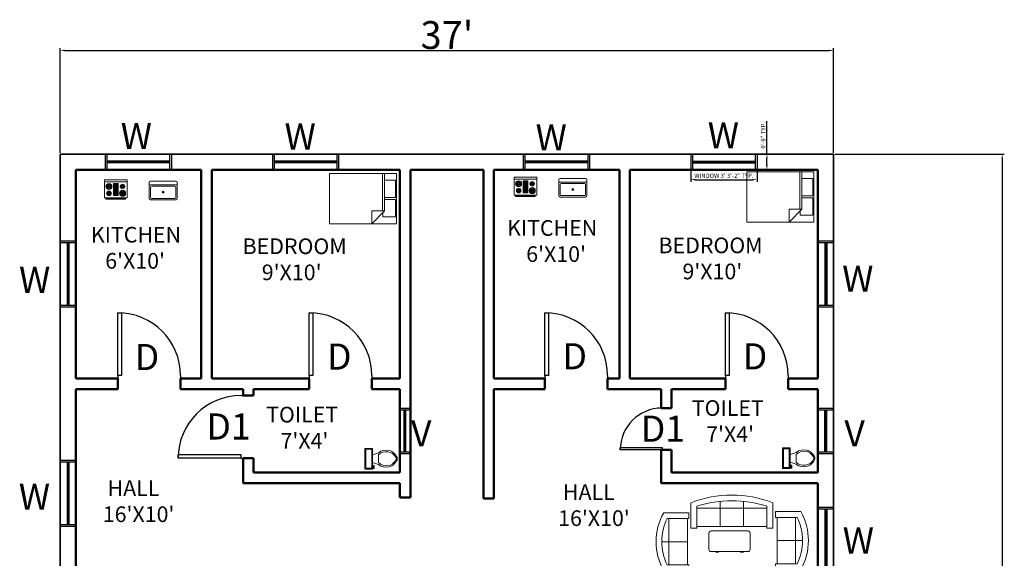
# Model space of a CAD drawing. Units: inches. Extents: x -25308 to -23933, y 10755 to 11996.
# Tile 4 of 6: x -25305 to -24739, y 11683 to 11992. Entities that reach past the tile are written whole.
import ezdxf

# ---------------------------------------------------------------- set-up
doc = ezdxf.new("R2010")
doc.units = ezdxf.units.IN
for name, color, linetype, lineweight in [('A-ANNO-DIMS', 2, 'Continuous', 18), ('A-ANNO-SYMB', 3, 'Continuous', 18), ('A-AREA-IDEN', 7, 'Continuous', 18), ('A-DOOR', 3, 'Continuous', 25), ('A-FLOR-FIXT', 8, 'Continuous', 18), ('A-FURN', 8, 'Continuous', 18), ('A-GLAZ', 4, 'Continuous', 25), ('A-WALL', 7, 'Continuous', 50), ('C-PROP', 30, 'Continuous', 35)]:
    doc.layers.add(name, color=color, linetype=linetype, lineweight=lineweight)
doc.styles.get("Standard").update_dxf_attribs({"font": 'arial.ttf'})
doc.dimstyles.new('ISO-25', dxfattribs={"dimtxt": 2.5, "dimasz": 2.5, "dimexe": 1.25, "dimexo": 0.625, "dimtad": 1, "dimdec": 0, "dimlunit": 3, "dimtxsty": 'Standard', "dimcen": 2.5, "dimadec": 0, "dimazin": 0, "dimtfac": 1, "dimtdec": 0, "dimtmove": 0, "dimatfit": 3, "dimfxl": 1, "dimarcsym": 0})

# ---------------------------------------------------------------- blocks, each defined once
blk = doc.blocks.new('*U8')
for p, q in [((0, 0), (0, -100)), ((750, 0), (750, -100))]:
    blk.add_line(p, q)
blk.add_lwpolyline([(0, 0), (0, 750), (43.75, 750), (43.75, 0)], close=True)
blk.add_arc((0, 0), 750, 0, 90)
blk = doc.blocks.new('Desk - 30 x 60 in.')
for p, q in [((-26.999995, 0), (26.999995, 0)), ((-29.999995, -27), (-29.999995, -3)), ((29.999995, -3), (29.999995, -27)), ((26.999995, -30), (-26.999995, -30)), ((-20.000005, -30), (-20.000005, -31)), ((-20.000005, -31), (-16.000005, -31)), ((-16.000005, -31), (-16.000005, -30)), ((15.999995, -31), (15.999995, -30)), ((19.999995, -31), (15.999995, -31)), ((19.999995, -30), (19.999995, -31))]:
    blk.add_line(p, q)
for centre, start, end in [((-26.499995, -3.5), 98.1301, 171.8699), ((26.499995, -3.5), 8.130102, 81.8699), ((-26.499995, -26.5), 188.1301, 261.8699), ((26.499995, -26.5), 278.1301, 351.8699)]:
    blk.add_arc(centre, 3.535534, start, end)
blk = doc.blocks.new('Sofa - Roundback 7 ft.')
for p, q in [((-12.00002, -32.4421), (-12.00003, -6.5971)), ((11.99997, -32.4421), (11.99998, -6.5971)), ((-36.000027, -34), (-36.000027, -11.4696)), ((-35.999844, -13.3819), (35.9998, -13.3819)), ((35.99998, -34), (35.99998, -11.4696)), ((-36.000027, -32.4421), (35.99998, -32.4421))]:
    blk.add_line(p, q)
for points in [[(-36.000027, -34), (-42.000027, -34), (-42.000027, -8)], [(41.99998, -8), (41.99998, -34), (35.99998, -34)]]:
    blk.add_lwpolyline(points)
for centre, radius, start, end in [((0, -114.25), 114.25, 68.43141, 111.5686), ((-0.00001, -127.1968), 121.1968, 72.72033, 107.2797)]:
    blk.add_arc(centre, radius, start, end)
blk = doc.blocks.new('Sofa - Roundback Loveseat 5 ft.')
for p, q in [((0, -32.44198), (0, -5.99998)), ((-24, -33.99998), (-24, -11.46958)), ((-23.9998, -13.38178), (23.99986, -13.38178)), ((24.00004, -33.99998), (24.00004, -11.46958)), ((-24, -32.44198), (24.00004, -32.44198))]:
    blk.add_line(p, q)
for points in [[(-24, -33.99998), (-30, -33.99998), (-30, -7.99998)], [(30.00004, -7.99998), (30.00004, -33.99998), (24.00004, -33.99998)]]:
    blk.add_lwpolyline(points)
for centre, radius, start, end in [((0, -60.24998), 60.24998, 60.13715, 119.8628), ((0, -61.38438), 55.38444, 64.32083, 115.6792)]:
    blk.add_arc(centre, radius, start, end)
blk = doc.blocks.new('Bed - Queen')
for p, q in [((0, -80.00003), (0, 0)), ((0, 0), (59.99999, 0)), ((59.99999, 0), (59.99999, -80.00003)), ((7.99999, -1.2), (28.79998, -1.2)), ((7.99999, -14.4), (7.99999, -1.2)), ((28.79998, -1.2), (28.79998, -14.4)), ((31.19999, -1.2), (51.99999, -1.2)), ((31.19999, -14.4), (31.19999, -1.2)), ((51.99999, -1.2), (51.99999, -16.4)), ((0, -14.4), (44.8, -14.4)), ((44.8, -16.8), (0, -16.8)), ((59.99999, -29.6), (44.8, -14.4)), ((44.8, -14.4), (44.8, -29.6)), ((51.99999, -16.4), (46.79936, -16.4)), ((44.8, -29.6), (59.99999, -29.6)), ((59.99999, -80.00003), (0, -80.00003))]:
    blk.add_line(p, q)
blk = doc.blocks.new('Range-Oven - 30 in top')
for p, q in [((0, -3), (30, -3)), ((12, -6), (18, -6)), ((13, -20), (13, -6)), ((14, -6), (14, -20)), ((15, -20), (15, -6)), ((16, -6), (16, -20)), ((17, -20), (17, -6)), ((6, -24), (6, -25)), ((8, -25), (8, -24)), ((18, -20), (12, -20)), ((22, -25), (22, -24)), ((24, -24), (24, -25))]:
    blk.add_line(p, q)
for points in [[(0, -24), (0, 0), (30, 0), (30, -24)], [(12, -21), (12, -5), (18, -5), (18, -21)], [(2, -26), (2, -25), (28, -25), (28, -26)]]:
    blk.add_lwpolyline(points, close=True)
for centre, radius in [((6, -9), 4), ((6, -9), 3), ((6, -9), 2), ((6, -9), 1), ((24, -9), 3), ((24, -9), 2), ((24, -9), 1), ((6, -18), 3), ((6, -18), 2), ((6, -18), 1), ((24, -18), 4), ((24, -18), 3), ((24, -18), 2), ((24, -18), 1)]:
    blk.add_circle(centre, radius)
blk = doc.blocks.new('Sink-single - 30 in top')
blk.add_line((-15, -3.999996), (15, -3.999996))
for points in [[(-13.5, 0), (13.5, 0)], [(-15, -18.499996), (-15, -1.5)], [(-13.5, -17.499996), (-13.5, -6.499996)], [(-12.5, -5.499996), (12.5, -5.499996)], [(13.5, -6.499996), (13.5, -17.499996)], [(15, -1.5), (15, -18.499996)], [(13.5, -19.999996), (-13.5, -19.999996)], [(12.5, -18.499996), (-12.5, -18.499996)]]:
    blk.add_lwpolyline(points)
for radius in [1, 0.5]:
    blk.add_circle((0, -11.999996), radius)
for centre, radius, start, end in [((-13.5, -1.5), 1.5, 90, 180), ((-12.5, -6.499996), 1, 90, 180), ((12.5, -6.499996), 1, 0, 90), ((13.5, -1.5), 1.5, 0, 90), ((-13.5, -18.499996), 1.5, 180, 270), ((-12.5, -17.499996), 1, 180, 270), ((12.5, -17.499996), 1, 270, 0), ((13.5, -18.499996), 1.5, 270, 0)]:
    blk.add_arc(centre, radius, start, end)
blk = doc.blocks.new('Toilet - top')
for p, q in [((-10, -8.5), (-8, -8.5)), ((-10, -9.5), (-10, -8.5)), ((-7, -9.5), (-10, -9.5)), ((-8, -8.5), (-8, -8)), ((-7, -8), (-7, -9.5)), ((-4, -8), (-6, -14)), ((4, -8), (6, -14)), ((9.5, -6), (9.5, -2)), ((4, -14), (-4, -14))]:
    blk.add_line(p, q)
blk.add_lwpolyline([(10.5, -8), (10.5, 0), (-10.5, 0), (-10.5, -8)], close=True)
for points in [[(-9.5, -2), (-9.5, -6)], [(8.5, -1), (-8.5, -1)], [(-8.5, -7), (8.5, -7)]]:
    blk.add_lwpolyline(points)
for centre, radius, start, end in [((-8.62, -1.88), 0.884, 81.8699, 188.1301), ((-8.62, -6.12), 0.884, 171.8699, 278.1301), ((8.62, -1.88), 0.884, 351.8699, 98.1301), ((8.62, -6.12), 0.884, 261.8699, 8.1301), ((3.52, -21.58), 12.17, 141.46911, 247.97143), ((4.2, -21.82), 11.33, 136.36773, 238.94682), ((-3.52, -21.58), 12.17, 292.02843, 38.53071), ((-4.2, -21.82), 11.33, 301.05301, 43.63209), ((0, -27.88), 4, 245.73182, 294.26817), ((0, -29), 4, 254.86053, 285.13947)]:
    blk.add_arc(centre, radius, start, end)
blk = doc.blocks.new('*D160')
at = {"layer": 'A-ANNO-DIMS', "color": 0, "lineweight": -2, "transparency": 16777216}
for p, q in [((-25281.44, 11915.75), (-25281.44, 11975.94)), ((-25278.94, 11974.69), (-24839.94, 11974.69)), ((-24837.44, 11915.75), (-24837.44, 11975.94))]:
    blk.add_line(p, q, dxfattribs=at)
at = {"layer": 'A-ANNO-DIMS', "color": 0, "transparency": 16777216}
for points in [[(-25278.94, 11975.11), (-25278.94, 11974.28), (-25281.44, 11974.69)], [(-24839.94, 11975.11), (-24839.94, 11974.28), (-24837.44, 11974.69)]]:
    blk.add_solid(points, dxfattribs=at)
at = {"layer": 'Defpoints', "color": 0, "transparency": 16777216}
for p in [(-24837.44, 11974.69), (-25281.44, 11915.12), (-24837.44, 11915.12)]:
    blk.add_point(p, dxfattribs=at)
at = {"layer": 'A-ANNO-DIMS', "color": 0, "transparency": 16777216, "insert": (-25059.44, 11983.49), "char_height": 2.5, "attachment_point": 5}
blk.add_mtext("{\\H6.4x;37'}", dxfattribs=at)
blk = doc.blocks.new('*D161')
at = {"layer": 'A-ANNO-DIMS', "color": 0, "lineweight": -2, "transparency": 16777216}
for p, q in [((-24836.82, 11915.12), (-24739.49, 11915.12)), ((-24740.74, 11912.62), (-24740.74, 10813.62)), ((-24836.82, 10811.12), (-24739.49, 10811.12))]:
    blk.add_line(p, q, dxfattribs=at)
at = {"layer": 'A-ANNO-DIMS', "color": 0, "transparency": 16777216}
for points in [[(-24741.15, 11912.62), (-24740.32, 11912.62), (-24740.74, 11915.12)], [(-24741.15, 10813.62), (-24740.32, 10813.62), (-24740.74, 10811.12)]]:
    blk.add_solid(points, dxfattribs=at)
at = {"layer": 'Defpoints', "color": 0, "transparency": 16777216}
for p in [(-24837.44, 11915.12), (-24837.44, 10811.12), (-24740.74, 10811.12)]:
    blk.add_point(p, dxfattribs=at)
at = {"layer": 'A-ANNO-DIMS', "color": 0, "transparency": 16777216, "insert": (-24749.53, 11363.12), "char_height": 2.5, "attachment_point": 5, "rotation": 90}
blk.add_mtext("{\\H6.4x;92'}", dxfattribs=at)
blk = doc.blocks.new('WIN-36-9IN')
for p, q in [((0, 9), (0, 0)), ((1, 9), (1, 0)), ((37, 9), (37, 0)), ((38, 9), (38, 0)), ((1, 5), (37, 5)), ((1, 4.5), (37, 4.5)), ((1, 4), (37, 4))]:
    blk.add_line(p, q)
blk = doc.blocks.new('VENT-24')
for p, q in [((0, 26), (9, 26)), ((0, 25), (9, 25)), ((4, 1), (4, 25)), ((4.5, 1), (4.5, 25)), ((5, 1), (5, 25)), ((0, 1), (9, 1)), ((0, 0), (9, 0))]:
    blk.add_line(p, q)
blk = doc.blocks.new('WIN-24-6IN')
for p, q in [((0, 26), (6, 26)), ((0, 25), (6, 25)), ((2.5, 1), (2.5, 25)), ((3, 1), (3, 25)), ((3.5, 1), (3.5, 25)), ((0, 1), (6, 1)), ((0, 0), (6, 0))]:
    blk.add_line(p, q)
blk = doc.blocks.new('*D182')
at = {"layer": 'A-ANNO-DIMS', "color": 0, "lineweight": -2, "transparency": 16777216}
for p, q in [((-24919.44, 11905.5), (-24919.44, 11899.17)), ((-24881.44, 11905.5), (-24881.44, 11899.17)), ((-24916.94, 11900.42), (-24883.94, 11900.42))]:
    blk.add_line(p, q, dxfattribs=at)
at = {"layer": 'A-ANNO-DIMS', "color": 0, "transparency": 16777216}
for points in [[(-24916.94, 11900.84), (-24916.94, 11900), (-24919.44, 11900.42)], [(-24883.94, 11900.84), (-24883.94, 11900), (-24881.44, 11900.42)]]:
    blk.add_solid(points, dxfattribs=at)
at = {"layer": 'Defpoints', "color": 0, "transparency": 16777216}
for p in [(-24919.44, 11906.12), (-24881.44, 11906.12), (-24881.44, 11900.42)]:
    blk.add_point(p, dxfattribs=at)
at = {"layer": 'A-ANNO-DIMS', "color": 0, "transparency": 16777216, "insert": (-24900.44, 11902.34), "char_height": 2.5, "attachment_point": 5}
blk.add_mtext('WINDOW 3\' 3\'-2" TYP.', dxfattribs=at)
blk = doc.blocks.new('*D183')
at = {"layer": 'A-ANNO-DIMS', "color": 0, "lineweight": -2, "transparency": 16777216}
for p, q in [((-24875.74, 11915.12), (-24875.74, 11934.11)), ((-24880.82, 11915.12), (-24874.49, 11915.12)), ((-24875.74, 11908.62), (-24875.74, 11912.62)), ((-24880.82, 11906.12), (-24874.49, 11906.12))]:
    blk.add_line(p, q, dxfattribs=at)
at = {"layer": 'A-ANNO-DIMS', "color": 0, "transparency": 16777216}
for points in [[(-24876.16, 11912.62), (-24875.33, 11912.62), (-24875.74, 11915.12)], [(-24876.16, 11908.62), (-24875.33, 11908.62), (-24875.74, 11906.12)]]:
    blk.add_solid(points, dxfattribs=at)
at = {"layer": 'Defpoints', "color": 0, "transparency": 16777216}
for p in [(-24881.44, 11915.12), (-24875.74, 11915.12), (-24881.44, 11906.12)]:
    blk.add_point(p, dxfattribs=at)
at = {"layer": 'A-ANNO-DIMS', "color": 0, "transparency": 16777216, "insert": (-24877.65, 11925.87), "char_height": 2.5, "attachment_point": 5, "rotation": 90}
blk.add_mtext('0\'-9" TYP.', dxfattribs=at)

msp = doc.modelspace()

# ---------------------------------------------------------------- linework, layer by layer
at = {"layer": 'A-WALL'}
for p, q in [((-25272.44, 11906.12), (-25200.44, 11906.12)), ((-25272.44, 11786.12), (-25272.44, 11906.12)), ((-25200.44, 11786.12), (-25200.44, 11906.12)), ((-25194.44, 11786.12), (-25194.44, 11906.12)), ((-25194.44, 11906.12), (-25086.44, 11906.12)), ((-25086.44, 11786.12), (-25086.44, 11906.12)), ((-25080.44, 11906.12), (-25038.44, 11906.12)), ((-25080.44, 11717.94), (-25080.44, 11906.12)), ((-25038.44, 11906.12), (-25038.44, 11717.22)), ((-25032.44, 11906.12), (-25032.44, 11786.12)), ((-25032.44, 11906.12), (-24960.44, 11906.12)), ((-24960.44, 11906.12), (-24960.44, 11786.12)), ((-24960.44, 11906.12), (-24960.44, 11786.12)), ((-24960.44, 11906.12), (-24960.44, 11786.12)), ((-24960.44, 11906.12), (-24960.44, 11786.12)), ((-24954.44, 11906.12), (-24954.44, 11786.12)), ((-24954.44, 11906.12), (-24954.44, 11786.12)), ((-24954.44, 11906.12), (-24954.44, 11786.12)), ((-24954.44, 11906.12), (-24954.44, 11786.12)), ((-24954.44, 11906.12), (-24846.44, 11906.12)), ((-24846.44, 11906.12), (-24846.44, 11786.12)), ((-25272.44, 11786.12), (-25248.38, 11786.12)), ((-25248.38, 11786.12), (-25248.38, 11780.12)), ((-25212.38, 11786.12), (-25212.38, 11780.12)), ((-25212.38, 11786.12), (-25200.44, 11786.12)), ((-25194.44, 11786.12), (-25138.54, 11786.12)), ((-25138.54, 11786.12), (-25138.54, 11780.12)), ((-25102.54, 11786.12), (-25102.54, 11780.12)), ((-25102.54, 11786.12), (-25086.44, 11786.12)), ((-25032.44, 11786.12), (-25003.22, 11786.12)), ((-25003.22, 11786.12), (-25003.22, 11780.12)), ((-24967.22, 11786.12), (-24967.22, 11780.12)), ((-24967.22, 11786.12), (-24960.44, 11786.12)), ((-24954.44, 11786.12), (-24899.58, 11786.12)), ((-24899.58, 11786.12), (-24899.58, 11780.12)), ((-24863.58, 11786.12), (-24863.58, 11780.12)), ((-24863.58, 11786.12), (-24846.44, 11786.12)), ((-25272.44, 11780.12), (-25248.38, 11780.12)), ((-25272.44, 11660.12), (-25272.44, 11780.12)), ((-25212.38, 11780.12), (-25176.44, 11780.12)), ((-25176.44, 11776.42), (-25176.44, 11780.12)), ((-25176.44, 11776.42), (-25176.44, 11780.12)), ((-25176.44, 11776.42), (-25176.44, 11780.12)), ((-25170.44, 11780.12), (-25138.54, 11780.12)), ((-25170.44, 11776.42), (-25170.44, 11780.12)), ((-25170.44, 11776.42), (-25170.44, 11780.12)), ((-25170.44, 11776.42), (-25170.44, 11780.12)), ((-25102.54, 11780.12), (-25086.44, 11780.12)), ((-25086.44, 11732.12), (-25086.44, 11780.12)), ((-25032.44, 11780.12), (-25003.22, 11780.12)), ((-25032.44, 11780.12), (-25032.44, 11717.22)), ((-24967.22, 11780.12), (-24936.44, 11780.12)), ((-24936.44, 11780.12), (-24936.44, 11769.19)), ((-24936.44, 11780.12), (-24936.44, 11769.19)), ((-24936.44, 11780.12), (-24936.44, 11769.19)), ((-24936.44, 11780.12), (-24936.44, 11769.19)), ((-24930.44, 11780.12), (-24930.44, 11769.19)), ((-24930.44, 11780.12), (-24930.44, 11769.19)), ((-24930.44, 11780.12), (-24930.44, 11769.19)), ((-24930.44, 11780.12), (-24930.44, 11769.19)), ((-24930.44, 11780.12), (-24899.58, 11780.12)), ((-24863.58, 11780.12), (-24846.44, 11780.12)), ((-24846.44, 11780.12), (-24846.44, 11732.12)), ((-25176.44, 11776.42), (-25170.44, 11776.42)), ((-24936.44, 11769.19), (-24930.44, 11769.19)), ((-24936.44, 11745.19), (-24930.44, 11745.19)), ((-24936.44, 11745.19), (-24936.44, 11726.12)), ((-24936.44, 11745.19), (-24936.44, 11726.12)), ((-24936.44, 11745.19), (-24936.44, 11726.12)), ((-24936.44, 11745.19), (-24936.44, 11726.12)), ((-24930.44, 11745.19), (-24930.44, 11732.12)), ((-24930.44, 11745.19), (-24930.44, 11732.12)), ((-24930.44, 11745.19), (-24930.44, 11732.12)), ((-24930.44, 11745.19), (-24930.44, 11732.12)), ((-25176.44, 11726.12), (-25176.44, 11740.42)), ((-25176.44, 11726.12), (-25176.44, 11740.42)), ((-25176.44, 11726.12), (-25176.44, 11740.42)), ((-25176.44, 11740.42), (-25170.44, 11740.42)), ((-25170.44, 11732.12), (-25170.44, 11740.42)), ((-25170.44, 11732.12), (-25170.44, 11740.42)), ((-25170.44, 11732.12), (-25170.44, 11740.42)), ((-25170.44, 11732.12), (-25086.44, 11732.12)), ((-24930.44, 11732.12), (-24846.44, 11732.12)), ((-25176.44, 11726.12), (-25086.44, 11726.12)), ((-25086.44, 11717.94), (-25086.44, 11726.12)), ((-24936.44, 11726.12), (-24846.44, 11726.12)), ((-24846.44, 11726.12), (-24846.44, 11660.12)), ((-25086.44, 11717.94), (-25080.44, 11717.94)), ((-25038.44, 11717.22), (-25032.44, 11717.22))]:
    msp.add_line(p, q, dxfattribs=at)
at = {"layer": 'C-PROP'}
for p, q in [((-25281.44, 11915.12), (-24837.44, 11915.12)), ((-25281.44, 10811.12), (-25281.44, 11915.12)), ((-24837.44, 11915.12), (-24837.44, 10811.12))]:
    msp.add_line(p, q, dxfattribs=at)

# ---------------------------------------------------------------- block references
at = {"layer": 'A-DOOR', "xscale": 0.0480000000000013, "yscale": 0.0480000000000013, "zscale": 0.0480000000000013}
for p in [(-25248.38, 11787.92), (-25138.54, 11787.92), (-25003.22, 11787.92), (-24899.58, 11787.92)]:
    msp.add_blockref('*U8', p, dxfattribs=at)
at = {"layer": 'A-DOOR', "rotation": 90}
for p, xscale, yscale, zscale in [((-25177.73, 11740.42), 0.0480000000000013, 0.0480000000000013, 0.0480000000000013), ((-24935.92, 11745.16), 0.0320853447088354, 0.0320853447088354, 0.0320853447088354)]:
    msp.add_blockref('*U8', p, dxfattribs=dict(at, xscale=xscale, yscale=yscale, zscale=zscale))
at = {"layer": 'A-FLOR-FIXT'}
for name, p, xscale, yscale, zscale in [('Range-Oven - 30 in top', (-25256.04, 11900.41), 0.4338097128947254, 0.4338097128947254, 0.4338097128947254), ('Sink-single - 30 in top', (-25222.36, 11899.64), 0.5374838416175965, 0.5374838416175965, 0.5374838416175965), ('Range-Oven - 30 in top', (-25020.89, 11901.95), 0.4338097128947254, 0.4338097128947254, 0.4338097128947254), ('Sink-single - 30 in top', (-24987.21, 11901.18), 0.5374838416175965, 0.5374838416175965, 0.5374838416175965)]:
    msp.add_blockref(name, p, dxfattribs=dict(at, xscale=xscale, yscale=yscale, zscale=zscale))
at = {"layer": 'A-FLOR-FIXT', "xscale": 0.5659332238665749, "yscale": 0.5659332238665749, "zscale": 0.5659332238665749, "rotation": 90}
for p in [(-25106.6, 11740.14), (-24866.87, 11740.37)]:
    msp.add_blockref('Toilet - top', p, dxfattribs=at)
at = {"layer": 'A-FURN'}
for name, p, xscale, yscale, zscale, rotation in [('Bed - Queen', (-25088.38, 11904.02), 0.4812808282186369, 0.4812808282186369, 0.4812808282186369, 270), ('Bed - Queen', (-24848.83, 11904.96), 0.4812808282186369, 0.4812808282186369, 0.4812808282186369, 270), ('Sofa - Roundback Loveseat 5 ft.', (-24939.4, 11692.47), 0.5553292889469988, 0.5553292889469988, 0.5553292889469988, 89.99999999999999), ('Sofa - Roundback Loveseat 5 ft.', (-24851.93, 11693.12), 0.5553292889469988, 0.5553292889469988, 0.5553292889469988, 270)]:
    msp.add_blockref(name, p, dxfattribs=dict(at, xscale=xscale, yscale=yscale, zscale=zscale, rotation=rotation))
for name, p, xscale, yscale, zscale in [('Sofa - Roundback 7 ft.', (-24895.88, 11719.27), 0.559663641165008, 0.559663641165008, 0.559663641165008), ('Desk - 30 x 60 in.', (-24897.18, 11698.61), 0.3949565101416468, 0.3949565101416468, 0.3949565101416468)]:
    msp.add_blockref(name, p, dxfattribs=dict(at, xscale=xscale, yscale=yscale, zscale=zscale))
at = {"layer": 'A-GLAZ'}
for p, rotation in [((-25217.44, 11915.12), 180), ((-25121.44, 11915.12), 180), ((-24977.44, 11915.12), 180), ((-25281.44, 11865.12), 270.0000000000315), ((-24846.44, 11865.12), 270.0000000000211), ((-25281.44, 11739.12), 270.0000000000211), ((-24846.44, 11712.12), 270.0000000000173)]:
    msp.add_blockref('WIN-36-9IN', p, dxfattribs=dict(at, rotation=rotation))
for name, p in [('WIN-36-9IN', (-24919.44, 11906.12)), ('WIN-24-6IN', (-25086.44, 11743.12)), ('VENT-24', (-24846.44, 11743.12))]:
    msp.add_blockref(name, p, dxfattribs=at)

# ---------------------------------------------------------------- texts
at = {"layer": 'A-ANNO-SYMB', "char_height": 15, "attachment_point": 1}
for s, insert in [('{W}', (-25246.71, 11933.06)), ('{W}', (-25152.65, 11932.69)), ('{W}', (-25008.55, 11932.23)), ('{W}', (-24909.74, 11933.41)), ('{W}', (-25305.08, 11850.4)), ('{W}', (-24832.56, 11851)), ('{D}', (-25238.67, 11806.04)), ('{D}', (-25128.29, 11806.28)), ('{D}', (-24993.1, 11806.48)), ('{D}', (-24889.64, 11806.41)), ('{D1}', (-25197.5, 11766.15)), ('{V}', (-25080.07, 11762.2)), ('{D1}', (-24948.14, 11764.86)), ('{V}', (-24831.31, 11762.2)), ('{W}', (-25305.21, 11725.81)), ('{W}', (-24832.26, 11700.65))]:
    msp.add_mtext_dynamic_manual_height_columns(s, width=1123.2502, gutter_width=12.5, heights=[0], dxfattribs=dict(at, insert=insert))
at = {"layer": 'A-AREA-IDEN', "char_height": 9, "attachment_point": 1}
for s, heights, insert in [("{  KITCHEN\\P      6'X10'}", [0], (-25030.42, 11877.18)), ("{KITCHEN\\P   6'X10'}", [0], (-25263.83, 11873.3)), ("{BEDROOM\\P    9'X10'}", [0], (-25176.72, 11866.68)), ("{BEDROOM\\P     9'X10'}", [0], (-24937.98, 11867.18)), ("{TOILET\\P   7'X4'}", [0], (-24918.88, 11773.75)), ("{TOILET\\P   7'X4'}", [0], (-25163.21, 11769.96)), ("{ HALL^J16'X10'}", [24.41], (-25256.98, 11727.74)), ("{           HALL\\P          16'X10'}", [0], (-25023.09, 11725.48))]:
    msp.add_mtext_dynamic_manual_height_columns(s, width=1489.8169, gutter_width=12.5, heights=heights, dxfattribs=dict(at, insert=insert))

# ---------------------------------------------------------------- dimensions: what is measured, and where the dimension line sits
at = {"layer": 'A-ANNO-DIMS'}
for base, p1, p2, text, override, picture, middle in [((-24837.44, 11974.69), (-25281.44, 11915.12), (-24837.44, 11915.12), '{\\H6.4x;<>}', {"dimclrd": 0, "dimclre": 0, "dimclrt": 0}, '*D160', (-25059.44, 11983.49)), ((-24881.44, 11900.42), (-24919.44, 11906.12), (-24881.44, 11906.12), "WINDOW 3' <> TYP.", {"dimdec": 1, "dimlfac": 1, "dimrnd": 0, "dimzin": 1, "dimdsep": 46, "dimlunit": 4, "dimfrac": 2}, '*D182', (-24900.44, 11902.34))]:
    dim = msp.add_linear_dim(base=base, p1=p1, p2=p2, text=text, dimstyle='ISO-25', override=override, dxfattribs=at)
    dim.commit()
    dim.dimension.update_dxf_attribs({"geometry": picture, "text_midpoint": middle})
for base, p1, p2, text, override, picture, middle in [((-24875.74, 11915.12), (-24881.44, 11906.12), (-24881.44, 11915.12), '<> TYP.', {"dimdec": 1, "dimlfac": 1, "dimrnd": 0, "dimzin": 1, "dimdsep": 46, "dimlunit": 4, "dimfrac": 2}, '*D183', (-24877.65, 11925.87)), ((-24740.74, 10811.12), (-24837.44, 11915.12), (-24837.44, 10811.12), '{\\H6.4x;<>}', {"dimclrd": 0, "dimclre": 0, "dimclrt": 0}, '*D161', (-24749.53, 11363.12))]:
    dim = msp.add_linear_dim(base=base, p1=p1, p2=p2, angle=90, text=text, dimstyle='ISO-25', override=override, dxfattribs=at)
    dim.commit()
    dim.dimension.update_dxf_attribs({"geometry": picture, "text_midpoint": middle})

doc.saveas('drawing.dxf')
